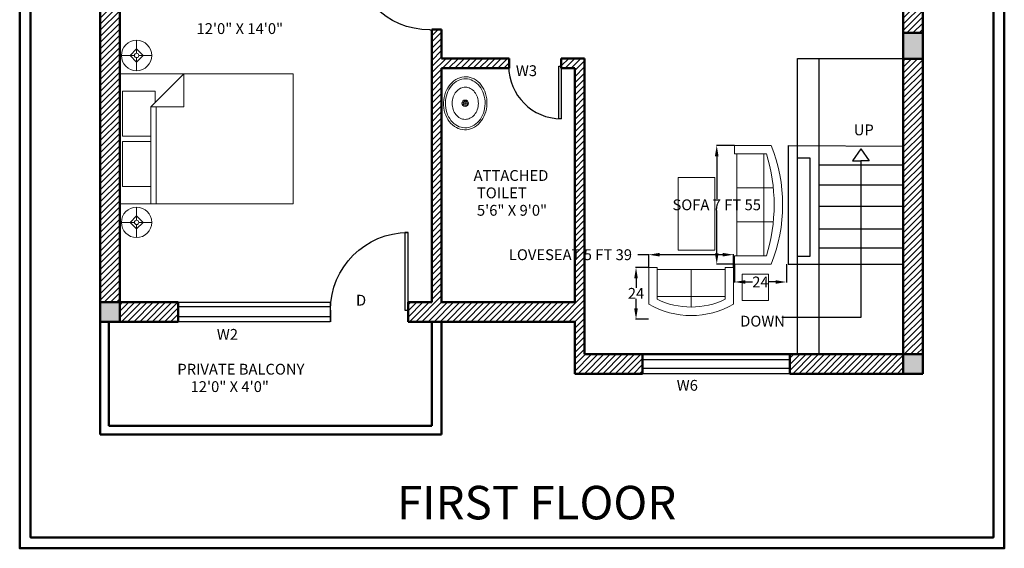
# Model space of a CAD drawing. Units: inches. Extents: x -25 to 429, y -18 to 847.
# Tile 1 of 3: x -25 to 429, y -18 to 226. Entities that reach past the tile are written whole.
import ezdxf

# ---------------------------------------------------------------- set-up
doc = ezdxf.new("R2010")
doc.units = ezdxf.units.IN
doc.header["$MEASUREMENT"] = 0
for name, color, linetype, lineweight in [('A-ANNO-DIMS', 2, 'Continuous', 18), ('A-ANNO-TEXT', 3, 'Continuous', 25), ('A-ANNO-TTLB', 7, 'Continuous', 50), ('A-AREA-IDEN', 7, 'Continuous', 25), ('A-DOOR', 4, 'Continuous', 25), ('A-FLOR-FIXT', 8, 'Continuous', 18), ('A-FLOR-STRS', 3, 'Continuous', 25), ('A-FURN', 8, 'Continuous', 18), ('A-GLAZ', 4, 'Continuous', 25), ('A-WALL', 7, 'Continuous', 50), ('A-WALL-FILL', 18, 'Continuous', 13), ('A-WALL-PATT', 252, 'Continuous', 13)]:
    doc.layers.add(name, color=color, linetype=linetype, lineweight=lineweight)
doc.styles.get("Standard").update_dxf_attribs({"font": 'arial.ttf'})
doc.dimstyles.get("Standard").update_dxf_attribs({"dimtxt": 5, "dimasz": 5, "dimexe": 0.18, "dimexo": 0.0625, "dimgap": 0.09, "dimtad": 0, "dimtih": 1, "dimtoh": 1, "dimdec": 1, "dimzin": 0, "dimdsep": 46, "dimlunit": 4, "dimtxsty": 'Standard', "dimcen": 0.09, "dimadec": 0, "dimazin": 0, "dimtfac": 1, "dimtdec": 1, "dimtofl": 0, "dimtmove": 0, "dimatfit": 3, "dimfxl": 1, "dimtolj": 1, "dimtzin": 0, "dimarcsym": 0})

# ---------------------------------------------------------------- blocks, each defined once
blk = doc.blocks.new('Sofa - Roundback 7 ft.')
for p, q in [((-12.00002, -32.4421), (-12.00003, -6.5971)), ((11.99997, -32.4421), (11.99998, -6.5971)), ((-36.000027, -34), (-36.000027, -11.4696)), ((-35.999844, -13.3819), (35.9998, -13.3819)), ((35.99998, -34), (35.99998, -11.4696)), ((-36.000027, -32.4421), (35.99998, -32.4421))]:
    blk.add_line(p, q)
for points in [[(-36.000027, -34), (-42.000027, -34), (-42.000027, -8)], [(41.99998, -8), (41.99998, -34), (35.99998, -34)]]:
    blk.add_lwpolyline(points)
for centre, radius, start, end in [((0, -114.25), 114.25, 68.43141, 111.5686), ((-0.00001, -127.1968), 121.1968, 72.72033, 107.2797)]:
    blk.add_arc(centre, radius, start, end)
blk = doc.blocks.new('Sofa - Roundback Loveseat 5 ft.')
for p, q in [((0, -32.44198), (0, -5.99998)), ((-24, -33.99998), (-24, -11.46958)), ((-23.9998, -13.38178), (23.99986, -13.38178)), ((24.00004, -33.99998), (24.00004, -11.46958)), ((-24, -32.44198), (24.00004, -32.44198))]:
    blk.add_line(p, q)
for points in [[(-24, -33.99998), (-30, -33.99998), (-30, -7.99998)], [(30.00004, -7.99998), (30.00004, -33.99998), (24.00004, -33.99998)]]:
    blk.add_lwpolyline(points)
for centre, radius, start, end in [((0, -60.24998), 60.24998, 60.13715, 119.8628), ((0, -61.38438), 55.38444, 64.32083, 115.6792)]:
    blk.add_arc(centre, radius, start, end)
blk = doc.blocks.new('Bed - Queen')
for p, q in [((0, -80.00003), (0, 0)), ((0, 0), (59.99999, 0)), ((59.99999, 0), (59.99999, -80.00003)), ((7.99999, -1.2), (28.79998, -1.2)), ((7.99999, -14.4), (7.99999, -1.2)), ((28.79998, -1.2), (28.79998, -14.4)), ((31.19999, -1.2), (51.99999, -1.2)), ((31.19999, -14.4), (31.19999, -1.2)), ((51.99999, -1.2), (51.99999, -16.4)), ((0, -14.4), (44.8, -14.4)), ((44.8, -16.8), (0, -16.8)), ((59.99999, -29.6), (44.8, -14.4)), ((44.8, -14.4), (44.8, -29.6)), ((51.99999, -16.4), (46.79936, -16.4)), ((44.8, -29.6), (59.99999, -29.6)), ((59.99999, -80.00003), (0, -80.00003))]:
    blk.add_line(p, q)
blk = doc.blocks.new('Lamp - Table')
for p, q in [((0, 7), (0, 1)), ((-1, 0), (-7, 0)), ((0, 3), (-3, 0)), ((-3, 0), (0, -3)), ((3, 0), (0, 3)), ((0, -3), (3, 0)), ((1, 0), (7, 0)), ((0, -1), (0, -7))]:
    blk.add_line(p, q)
for radius in [7, 1]:
    blk.add_circle((0, 0), radius)
blk = doc.blocks.new('Sink - Oval top')
for p, q in [((-1, 0), (1, 0)), ((0, 1), (0, -1))]:
    blk.add_line(p, q)
for points in [[(-12.23, 0.39, 0.117634), (-11.46, -3.36, 0.104469), (-8.88, -6.8, 0.090016), (-5.08, -9.07, 0.08192), (-0.32, -10.02, 0.08192), (4.49, -9.38, 0.090016), (8.42, -7.36, 0.104469), (11.22, -4.09, 0.117634), (12.23, -0.39, 0.117634), (11.46, 3.36, 0.104469), (8.88, 6.8, 0.090016), (5.08, 9.07, 0.08192), (0.32, 10.02, 0.08192), (-4.49, 9.38, 0.090016), (-8.42, 7.36, 0.104469), (-11.22, 4.09, 0.117634)], [(-11.29, 0.16, 0.118622), (-10.52, -3.25, 0.104678), (-8.07, -6.36, 0.089562), (-4.54, -8.37, 0.081185), (-0.13, -9.15, 0.081185), (4.3, -8.49, 0.089562), (7.89, -6.58, 0.104678), (10.42, -3.55, 0.118622), (11.29, -0.16, 0.118622), (10.52, 3.25, 0.104678), (8.07, 6.36, 0.089562), (4.54, 8.37, 0.081185), (0.13, 9.15, 0.081185), (-4.3, 8.49, 0.089562), (-7.89, 6.58, 0.104678), (-10.42, 3.55, 0.118622)], [(-7.42, 0.08, 0.118283), (-6.91, -2.17, 0.104607), (-5.29, -4.21, 0.089718), (-2.97, -5.53, 0.081436), (-0.07, -6.04, 0.081436), (2.84, -5.59, 0.089718), (5.2, -4.33, 0.104607), (6.86, -2.32, 0.118283), (7.42, -0.08, 0.118283), (6.91, 2.17, 0.104607), (5.29, 4.21, 0.089718), (2.97, 5.53, 0.081436), (0.07, 6.04, 0.081436), (-2.84, 5.59, 0.089718), (-5.2, 4.33, 0.104607), (-6.86, 2.32, 0.118283)]]:
    blk.add_lwpolyline(points, format="xyb", close=True)
for radius in [1.5, 1]:
    blk.add_circle((0, 0), radius)
blk = doc.blocks.new('*U10')
for p, q in [((0, 0), (0, -6)), ((40, 0), (40, -6))]:
    blk.add_line(p, q)
blk.add_lwpolyline([(0, 0), (0, 40), (1.75, 40), (1.75, 0)], close=True)
blk.add_arc((0, 0), 40, 0, 90)
blk = doc.blocks.new('*D19')
at = {"layer": 'A-ANNO-DIMS', "color": 0, "lineweight": -2, "ltscale": 0.5, "transparency": 16777216}
for p, q in [((304.74, 168.34), (296.4, 168.34)), ((296.58, 163.34), (296.58, 143.62)), ((296.58, 118.55), (296.58, 138.27)), ((304.74, 113.55), (296.4, 113.55))]:
    blk.add_line(p, q, dxfattribs=at)
at = {"layer": 'A-ANNO-DIMS', "color": 0, "lineweight": 100, "ltscale": 0.5, "transparency": 16777216}
for points in [[(295.75, 163.34), (297.41, 163.34), (296.58, 168.34)], [(295.75, 118.55), (297.41, 118.55), (296.58, 113.55)]]:
    blk.add_solid(points, dxfattribs=at)
at = {"layer": 'Defpoints', "color": 0, "lineweight": 100, "ltscale": 0.5, "transparency": 16777216}
for p in [(304.8, 168.34), (296.58, 113.55), (304.8, 113.55)]:
    blk.add_point(p, dxfattribs=at)
at = {"layer": 'A-ANNO-DIMS', "color": 0, "ltscale": 0.5, "transparency": 16777216, "insert": (296.58, 140.94), "char_height": 5, "attachment_point": 5}
blk.add_mtext('\\A1;SOFA 7 FT 55', dxfattribs=at)
blk = doc.blocks.new('*D20')
at = {"layer": 'A-ANNO-DIMS', "color": 0, "lineweight": -2, "ltscale": 0.5, "transparency": 16777216}
for p, q in [((304.8, 113.48), (304.8, 105.15)), ((328.72, 113.48), (328.72, 105.15)), ((309.8, 105.33), (313.05, 105.33)), ((323.72, 105.33), (320.46, 105.33))]:
    blk.add_line(p, q, dxfattribs=at)
at = {"layer": 'A-ANNO-DIMS', "color": 0, "lineweight": 100, "ltscale": 0.5, "transparency": 16777216}
for points in [[(309.8, 106.16), (309.8, 104.49), (304.8, 105.33)], [(323.72, 106.16), (323.72, 104.49), (328.72, 105.33)]]:
    blk.add_solid(points, dxfattribs=at)
at = {"layer": 'Defpoints', "color": 0, "lineweight": 100, "ltscale": 0.5, "transparency": 16777216}
for p in [(304.8, 113.55), (328.72, 113.55), (328.72, 105.33)]:
    blk.add_point(p, dxfattribs=at)
at = {"layer": 'A-ANNO-DIMS', "color": 0, "ltscale": 0.5, "transparency": 16777216, "insert": (316.76, 105.33), "char_height": 5, "attachment_point": 5}
blk.add_mtext('\\A1;24', dxfattribs=at)
blk = doc.blocks.new('*D23')
at = {"layer": 'A-ANNO-DIMS', "color": 0, "lineweight": -2, "ltscale": 0.5, "transparency": 16777216}
for p, q in [((265.21, 117.91), (260.21, 117.91)), ((265.21, 112.1), (265.21, 118.09)), ((299.35, 117.91), (270.21, 117.91)), ((304.35, 112.1), (304.35, 118.09))]:
    blk.add_line(p, q, dxfattribs=at)
at = {"layer": 'A-ANNO-DIMS', "color": 0, "lineweight": 100, "ltscale": 0.5, "transparency": 16777216}
for points in [[(270.21, 118.74), (270.21, 117.08), (265.21, 117.91)], [(299.35, 118.74), (299.35, 117.08), (304.35, 117.91)]]:
    blk.add_solid(points, dxfattribs=at)
at = {"layer": 'Defpoints', "color": 0, "lineweight": 100, "ltscale": 0.5, "transparency": 16777216}
for p in [(265.21, 117.91), (265.21, 112.04), (304.35, 112.04)]:
    blk.add_point(p, dxfattribs=at)
at = {"layer": 'A-ANNO-DIMS', "color": 0, "ltscale": 0.5, "transparency": 16777216, "insert": (229.08, 117.91), "char_height": 5, "attachment_point": 5}
blk.add_mtext('\\A1;LOVESEAT 5 FT 39', dxfattribs=at)
blk = doc.blocks.new('*D24')
at = {"layer": 'A-ANNO-DIMS', "color": 0, "lineweight": -2, "ltscale": 0.5, "transparency": 16777216}
for p, q in [((265.15, 112.04), (259.16, 112.04)), ((259.34, 107.04), (259.34, 102.68)), ((259.34, 93.12), (259.34, 97.48)), ((265.15, 88.12), (259.16, 88.12))]:
    blk.add_line(p, q, dxfattribs=at)
at = {"layer": 'A-ANNO-DIMS', "color": 0, "lineweight": 100, "ltscale": 0.5, "transparency": 16777216}
for points in [[(258.5, 107.04), (260.17, 107.04), (259.34, 112.04)], [(258.5, 93.12), (260.17, 93.12), (259.34, 88.12)]]:
    blk.add_solid(points, dxfattribs=at)
at = {"layer": 'Defpoints', "color": 0, "lineweight": 100, "ltscale": 0.5, "transparency": 16777216}
for p in [(265.21, 112.04), (259.34, 88.12), (265.21, 88.12)]:
    blk.add_point(p, dxfattribs=at)
at = {"layer": 'A-ANNO-DIMS', "color": 0, "ltscale": 0.5, "transparency": 16777216, "insert": (259.34, 100.08), "char_height": 5, "attachment_point": 5}
blk.add_mtext('\\A1;24', dxfattribs=at)

msp = doc.modelspace()

# ---------------------------------------------------------------- hatches: boundary and pattern name
at = {"layer": 'A-WALL-FILL'}
h = msp.add_hatch(color=256, dxfattribs=at)
h.dxf.hatch_style = 1
h.paths.add_polyline_path([(169.63, 272.99), (160.88, 272.99), (160.88, 263.99), (169.63, 263.99)])
h.paths.add_polyline_path([(21.13, 95.99), (12.13, 95.99), (12.13, 86.99), (21.13, 86.99)])
h.paths.add_polyline_path([(21.13, 272.99), (12.13, 272.99), (12.13, 263.99), (21.13, 263.99)])
h.paths.add_polyline_path([(391.63, 350.55), (382.63, 350.55), (382.63, 340.49), (391.63, 340.49)])
h.paths.add_polyline_path([(391.63, 71.99), (382.63, 71.99), (382.63, 62.99), (391.63, 62.99)])
h.paths.add_polyline_path([(391.63, 220.21), (382.63, 220.21), (382.63, 208.25), (391.63, 208.25)])
h.paths.add_polyline_path([(334.63, 449.99), (327.59, 449.99), (327.59, 440.99), (334.63, 440.99)])
h.paths.add_polyline_path([(391.63, 449.99), (382.63, 449.99), (382.63, 440.99), (391.63, 440.99)])
h.paths.add_polyline_path([(234.13, 449.99), (227.53, 449.99), (227.53, 440.99), (234.13, 440.99)])
h.paths.add_polyline_path([(172.34, 449.99), (165.13, 449.99), (165.13, 440.99), (172.34, 440.99)])
h.paths.add_polyline_path([(21.13, 449.99), (12.13, 449.99), (12.13, 440.99), (21.13, 440.99)])
at = {"layer": 'A-WALL-PATT'}
h = msp.add_hatch(dxfattribs=at)
h.set_pattern_fill('ANSI31', color=256, scale=16)
h.paths.add_polyline_path([(160.88, 272.99), (21.13, 272.99), (21.13, 263.99), (105.02, 263.99), (160.88, 263.99)])
h.paths.add_polyline_path([(169.63, 340.49), (199.38, 340.49), (199.38, 344.99), (169.63, 344.99), (169.63, 440.99), (165.13, 440.99), (165.13, 313.72), (169.63, 313.72)])
h.paths.add_polyline_path([(21.13, 440.99), (12.13, 440.99), (12.13, 272.99), (21.13, 272.99), (21.13, 299.31)])
h.paths.add_polyline_path([(62.34, 449.99), (21.13, 449.99), (21.13, 440.99), (62.34, 440.99)])
h.paths.add_polyline_path([(165.13, 449.99), (130.96, 449.99), (130.96, 440.99), (165.13, 440.99)])
h.paths.add_polyline_path([(184.34, 449.99), (172.34, 449.99), (172.34, 440.99), (184.34, 440.99)])
h.paths.add_polyline_path([(227.53, 449.99), (215.51, 449.99), (215.51, 440.99), (227.53, 440.99)])
h.paths.add_polyline_path([(247.61, 449.99), (234.13, 449.99), (234.13, 440.99), (247.61, 440.99)])
h.paths.add_polyline_path([(327.59, 449.99), (316.24, 449.99), (316.24, 440.99), (327.59, 440.99)])
h.paths.add_polyline_path([(234.1, 407.15), (234.12, 440.99), (229.63, 440.99), (229.63, 344.99), (223.38, 344.99), (223.38, 340.49), (240.63, 340.49), (240.63, 344.99), (234.13, 344.99), (234.13, 387.57), (234.1, 387.57)])
h.paths.add_polyline_path([(334.63, 440.99), (330.13, 440.99), (330.13, 344.99), (276.63, 344.99), (276.63, 340.49), (339.1, 340.49), (339.1, 344.99), (334.63, 344.99)])
h.paths.add_polyline_path([(382.63, 449.99), (334.63, 449.99), (334.63, 440.99), (382.63, 440.99)])
h.paths.add_polyline_path([(382.63, 344.99), (375.1, 344.99), (375.1, 340.49), (382.63, 340.49)])
h.paths.add_polyline_path([(391.63, 340.49), (382.63, 340.49), (382.63, 325.05), (391.63, 325.05)])
h.paths.add_polyline_path([(391.63, 273.01), (382.63, 273.01), (382.63, 220.21), (391.63, 220.21)])
h.paths.add_polyline_path([(391.63, 208.25), (382.63, 208.25), (382.63, 71.99), (391.63, 71.99)])
h.paths.add_polyline_path([(382.63, 71.99), (330.34, 71.99), (330.34, 62.99), (382.63, 62.99)])
h.paths.add_polyline_path([(262.4, 71.99), (235.63, 71.99), (235.63, 208.49), (224.79, 208.49), (224.79, 203.99), (231.13, 203.99), (231.13, 95.99), (169.63, 95.99), (169.63, 203.99), (200.79, 203.99), (200.79, 208.49), (169.63, 208.49), (169.63, 221.76), (165.13, 221.76), (165.13, 95.99), (154.17, 95.99), (154.17, 86.99), (231.13, 86.99), (231.13, 62.99), (262.4, 62.99)])
h.paths.add_polyline_path([(48.08, 95.99), (21.13, 95.99), (21.13, 86.99), (48.08, 86.99)])
h.paths.add_polyline_path([(21.13, 263.99), (12.13, 263.99), (12.13, 95.99), (21.13, 95.99)])
h.paths.add_polyline_path([(169.63, 263.99), (165.13, 263.99), (165.13, 257.76), (169.63, 257.76)])
h.paths.add_polyline_path([(169.63, 277.72), (165.13, 277.72), (165.13, 272.99), (169.63, 272.99)])

# ---------------------------------------------------------------- linework, layer by layer
at = {"layer": 'A-ANNO-TTLB', "ltscale": 0.5}
for points in [[(-25.05, 846.91), (429.28, 846.91), (429.28, -17.53), (-25.05, -17.53)], [(-20.05, 841.91), (424.28, 841.91), (424.28, -12.53), (-20.05, -12.53)]]:
    msp.add_lwpolyline(points, close=True, dxfattribs=at)
at = {"layer": 'A-FLOR-STRS'}
for p, q in [((333.87, 71.99), (333.87, 208.49)), ((333.87, 208.49), (382.63, 208.49)), ((343.63, 208.49), (343.63, 71.99)), ((329.51, 168.31), (382.63, 168)), ((329.51, 168.31), (329.51, 113.51)), ((363.13, 166.71), (359.27, 161.19)), ((363.13, 166.71), (366.99, 161.19)), ((333.87, 162.59), (339.6, 162.59)), ((339.6, 162.59), (339.6, 117.14)), ((343.63, 159.36), (382.63, 159.36)), ((359.27, 161.19), (363.13, 161.19)), ((366.99, 161.19), (363.13, 161.19)), ((363.13, 161.19), (363.13, 96.6)), ((343.63, 150.08), (382.63, 150.08)), ((343.63, 140.24), (382.63, 140.24)), ((343.63, 129.86), (382.63, 129.86)), ((343.63, 121.04), (382.63, 121.04)), ((339.6, 117.14), (333.87, 117.14)), ((329.51, 113.55), (382.63, 113.55)), ((363.13, 96.6), (363.13, 89)), ((363.13, 89), (326.66, 89))]:
    msp.add_line(p, q, dxfattribs=at)
at = {"layer": 'A-FURN'}
for points in [[(278.82, 153.48), (295.68, 153.48), (295.68, 120.07), (278.82, 120.07)], [(308.31, 109.01), (320.45, 109.01), (320.45, 96.8), (308.31, 96.8)]]:
    msp.add_lwpolyline(points, close=True, dxfattribs=at)
at = {"layer": 'A-GLAZ'}
for points in [[(118.17, 86.99), (48.08, 86.99), (48.08, 95.99), (118.17, 95.99)], [(48.08, 94.02), (118.17, 94.02), (118.17, 89.18), (48.08, 89.18)], [(262.4, 71.99), (330.34, 71.99), (330.34, 62.99), (262.4, 62.99)], [(262.4, 69.62), (330.34, 69.62), (330.34, 65.36), (262.4, 65.36)]]:
    msp.add_lwpolyline(points, close=True, dxfattribs=at)
at = {"layer": 'A-WALL'}
for p, q in [((12.13, 449.99), (12.13, 86.99)), ((21.13, 449.99), (21.13, 86.99)), ((382.63, 273.01), (382.63, 62.99)), ((391.63, 273.01), (391.63, 62.99)), ((165.13, 221.76), (169.63, 221.76)), ((165.13, 221.76), (165.13, 95.99)), ((169.63, 221.76), (169.63, 208.49)), ((169.63, 208.49), (200.79, 208.49)), ((200.79, 203.99), (200.79, 208.49)), ((224.79, 208.49), (224.79, 203.99)), ((224.79, 208.49), (235.63, 208.49)), ((235.63, 208.49), (235.63, 71.99)), ((169.63, 203.99), (200.79, 203.99)), ((169.63, 203.99), (169.63, 95.99)), ((224.79, 203.99), (231.13, 203.99)), ((231.13, 203.99), (231.13, 95.99)), ((12.13, 95.99), (48.08, 95.99)), ((48.08, 95.99), (48.08, 86.99)), ((154.17, 86.99), (154.17, 95.99)), ((154.17, 95.99), (165.13, 95.99)), ((169.63, 95.99), (231.13, 95.99)), ((12.13, 86.99), (48.08, 86.99)), ((12.13, 86.99), (12.13, 34.99)), ((16.13, 86.99), (16.13, 38.99)), ((154.17, 86.99), (231.13, 86.99)), ((165.13, 86.99), (165.13, 38.99)), ((169.63, 86.99), (169.63, 34.99)), ((231.13, 86.99), (231.13, 62.99)), ((235.63, 71.99), (262.4, 71.99)), ((262.4, 71.99), (262.4, 62.99)), ((262.4, 71.99), (391.63, 71.99)), ((330.34, 62.99), (330.34, 71.99)), ((330.34, 71.83), (330.34, 62.83)), ((231.13, 62.99), (262.4, 62.99)), ((330.34, 62.99), (391.63, 62.99)), ((16.13, 38.99), (165.13, 38.99)), ((12.13, 34.99), (169.63, 34.99))]:
    msp.add_line(p, q, dxfattribs=at)
msp.add_lwpolyline([(382.63, 220.21), (391.63, 220.21), (391.63, 208.25), (382.63, 208.25)], close=True, dxfattribs=at)

# ---------------------------------------------------------------- block references
at = {"layer": 'A-DOOR'}
for p, xscale, yscale, zscale, rotation in [((164.21, 257.76), -0.9032110208705866, 0.9032110208705866, 0.9032110208705866, 90), ((224.79, 204.86), 0.6050896280768714, 0.6050896280768714, 0.6050896280768714, 180)]:
    msp.add_blockref('*U10', p, dxfattribs=dict(at, xscale=xscale, yscale=yscale, zscale=zscale, rotation=rotation))
at = {"layer": 'A-DOOR', "xscale": -0.89524410089764, "yscale": 0.89524410089764, "zscale": 0.89524410089764}
msp.add_blockref('*U10', (154.17, 92.36), dxfattribs=at)
at = {"layer": 'A-FLOR-FIXT', "rotation": 90}
msp.add_blockref('Sink - Oval top', (180.54, 187.76), dxfattribs=at)
at = {"layer": 'A-FURN', "rotation": 90}
for name, p in [('Lamp - Table', (28.87, 209.81)), ('Bed - Queen', (21.13, 141.39)), ('Lamp - Table', (28.87, 132.82))]:
    msp.add_blockref(name, p, dxfattribs=at)
at = {"layer": 'A-FURN', "xscale": 0.6523234445211493, "yscale": 0.6523234445211493, "zscale": 0.6523234445211493}
for name, p, rotation in [('Sofa - Roundback 7 ft.', (326.98, 140.94), 270), ('Sofa - Roundback Loveseat 5 ft.', (284.78, 89.86), 180)]:
    msp.add_blockref(name, p, dxfattribs=dict(at, rotation=rotation))

# ---------------------------------------------------------------- texts
at = {"layer": 'A-ANNO-TEXT', "ltscale": 0.5}
for s, height, p in [('W3', 5, (203.89, 200.3)), ('UP', 5, (359.81, 173)), ('D', 5, (130.13, 94.42)), ('DOWN', 5, (307.4, 84.77)), ('W2', 5, (65.9, 78.66)), ('W6', 5, (278.11, 55.16)), ('FIRST FLOOR', 15.4568, (149.02, -4.18))]:
    msp.add_text(s, height=height, dxfattribs=at).set_placement(p)
at = {"layer": 'A-AREA-IDEN', "ltscale": 0.5}
for s, p in [('    12\'0" X 14\'0"', (50.43, 219.72)), ('ATTACHED', (184.4, 151.96)), (' TOILET', (184.4, 143.93)), (' 5\'6" X 9\'0"', (184.4, 135.89)), ('PRIVATE BALCONY', (47.68, 62.59)), ('    12\'0" X 4\'0"', (47.68, 54.56))]:
    msp.add_text(s, height=5, dxfattribs=at).set_placement(p)

# ---------------------------------------------------------------- dimensions: what is measured, and where the dimension line sits
at = {"layer": 'A-ANNO-DIMS', "ltscale": 0.5}
for base, p1, p2, angle, text, picture, middle in [((296.58, 113.55), (304.8, 168.34), (304.8, 113.55), 270, 'SOFA 7 FT <>', '*D19', (296.58, 140.94)), ((265.21, 117.91), (304.35, 112.04), (265.21, 112.04), 180, 'LOVESEAT 5 FT <>', '*D23', (229.08, 117.91))]:
    dim = msp.add_linear_dim(base=base, p1=p1, p2=p2, angle=angle, text=text, dimstyle='Standard', override={"dimdec": 0, "dimrnd": 0, "dimzin": 0, "dimlunit": 2}, dxfattribs=at)
    dim.commit()
    dim.dimension.update_dxf_attribs({"geometry": picture, "text_midpoint": middle})
dim = msp.add_linear_dim(base=(259.34, 88.12), p1=(265.21, 112.04), p2=(265.21, 88.12), angle=270, dimstyle='Standard', override={"dimdec": 0, "dimrnd": 0, "dimzin": 0, "dimlunit": 2}, dxfattribs=at)
dim.commit()
dim.dimension.update_dxf_attribs({"geometry": '*D24', "text_midpoint": (259.34, 100.08)})
dim = msp.add_linear_dim(base=(328.72, 105.33), p1=(304.8, 113.55), p2=(328.72, 113.55), dimstyle='Standard', override={"dimdec": 0, "dimrnd": 0, "dimzin": 0, "dimlunit": 2}, dxfattribs=at)
dim.commit()
dim.dimension.update_dxf_attribs({"geometry": '*D20', "text_midpoint": (316.76, 105.33)})

doc.saveas('drawing.dxf')
